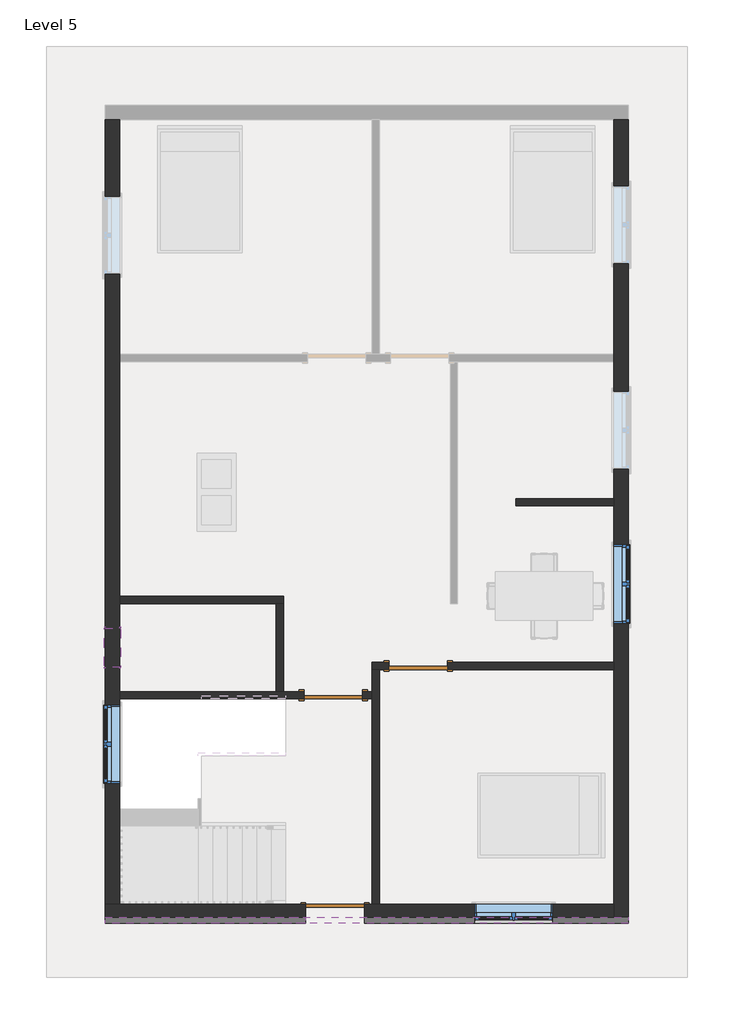
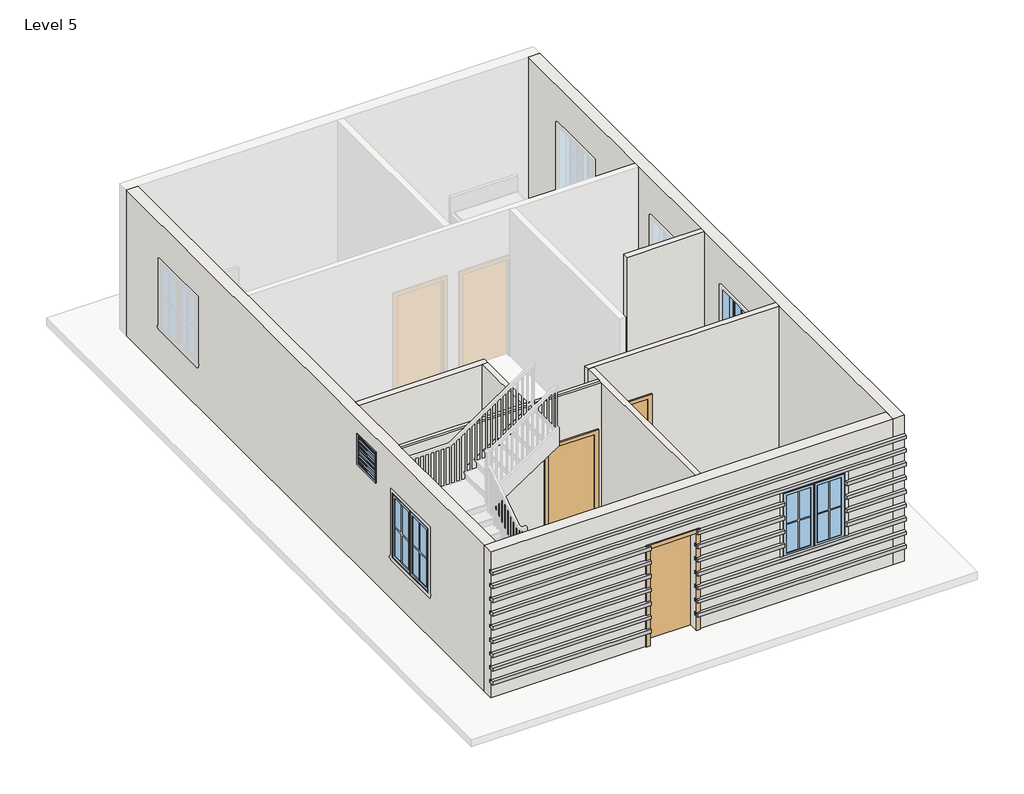
# One storey, part 1 of 3: 9 proxies, 9 walls, 4 windows, 3 doors.
"""IFC4 building model written with IfcOpenShell, lengths in millimetres."""

from ifc_helpers import new_model, si_unit, frame, origin, place, context, project, spatial, polyline, outline, extrude, faceted_brep, transform, mapped, element, save
from components import single_flush_door_3_17d80c48, single_flush_door_3_5e62189b, single_flush_door_3_89fc3733, window_casement_double_window_4_576b2d2c, window_f2d8fef0

model = new_model("IFC4")

# Units and contexts
model_context = context("Model", 3, world=origin())
ifc_project = project(units=[si_unit("LENGTHUNIT", "METRE", prefix="MILLI")], contexts=[model_context])

# Site, building, storey
site = spatial("IfcSite", under=ifc_project)
building = spatial("IfcBuilding", under=site)
storey = spatial("IfcBuildingStorey", under=building, Name="Level 5", Elevation=12649.2)

# Proxies
placement = place(None, origin())
element("IfcBuildingElementProxy", 1, Name="Reveal", ObjectType="Reveal", at=placement, inside=storey, context=model_context, shape_type="SweptSolid", body=[
    extrude(outline(polyline([(-2204.0617403, -6585.4426559), (-2204.0617403, -6677.5176559), (-5334.6117403, -6677.5176559), (-5334.6117403, -6585.4426559), (-2204.0617403, -6585.4426559)])), frame((0.0, 0.0, 12954.0), z_axis=(0.0, 0.0, 1.0), x_axis=(1.0, 0.0, 0.0)), (0.0, 0.0, 1.0), 67.7333333),
    extrude(outline(polyline([(2831.4882597, -6585.4426559), (2831.4882597, -6677.5176559), (-1289.6617403, -6677.5176559), (-1289.6617403, -6585.4426559), (2831.4882597, -6585.4426559)])), frame((0.0, 0.0, 12954.0), z_axis=(0.0, 0.0, 1.0), x_axis=(1.0, 0.0, 0.0)), (0.0, 0.0, 1.0), 67.7333333),
])
element("IfcBuildingElementProxy", 2, Name="Reveal", ObjectType="Reveal", at=placement, inside=storey, context=model_context, shape_type="SweptSolid", body=[
    extrude(outline(polyline([(-2204.0617403, -6585.4426559), (-2204.0617403, -6677.5176559), (-5334.6117403, -6677.5176559), (-5334.6117403, -6585.4426559), (-2204.0617403, -6585.4426559)])), frame((0.0, 0.0, 13240.4994231), z_axis=(0.0, 0.0, 1.0), x_axis=(1.0, 0.0, 0.0)), (0.0, 0.0, 1.0), 67.7333333),
    extrude(outline(polyline([(2831.4882597, -6585.4426559), (2831.4882597, -6677.5176559), (-1289.6617403, -6677.5176559), (-1289.6617403, -6585.4426559), (2831.4882597, -6585.4426559)])), frame((0.0, 0.0, 13240.4994231), z_axis=(0.0, 0.0, 1.0), x_axis=(1.0, 0.0, 0.0)), (0.0, 0.0, 1.0), 67.7333333),
])
element("IfcBuildingElementProxy", 3, Name="Reveal", ObjectType="Reveal", at=placement, inside=storey, context=model_context, shape_type="SweptSolid", body=[
    extrude(outline(polyline([(-2204.0617403, -6585.4426559), (-2204.0617403, -6677.5176559), (-5334.6117403, -6677.5176559), (-5334.6117403, -6585.4426559), (-2204.0617403, -6585.4426559)])), frame((0.0, 0.0, 13526.9988461), z_axis=(0.0, 0.0, 1.0), x_axis=(1.0, 0.0, 0.0)), (0.0, 0.0, 1.0), 67.7333333),
    extrude(outline(polyline([(2831.4882597, -6585.4426559), (2831.4882597, -6677.5176559), (-1289.6617403, -6677.5176559), (-1289.6617403, -6585.4426559), (2831.4882597, -6585.4426559)])), frame((0.0, 0.0, 13526.9988461), z_axis=(0.0, 0.0, 1.0), x_axis=(1.0, 0.0, 0.0)), (0.0, 0.0, 1.0), 67.7333333),
])
element("IfcBuildingElementProxy", 4, Name="Reveal", ObjectType="Reveal", at=placement, inside=storey, context=model_context, shape_type="SweptSolid", body=[
    extrude(outline(polyline([(431.1882597, -6585.4426559), (431.1882597, -6677.5176559), (-1289.6617403, -6677.5176559), (-1289.6617403, -6585.4426559), (431.1882597, -6585.4426559)])), frame((0.0, 0.0, 13813.4982692), z_axis=(0.0, 0.0, 1.0), x_axis=(1.0, 0.0, 0.0)), (0.0, 0.0, 1.0), 67.7333333),
    extrude(outline(polyline([(-2204.0617403, -6585.4426559), (-2204.0617403, -6677.5176559), (-5334.6117403, -6677.5176559), (-5334.6117403, -6585.4426559), (-2204.0617403, -6585.4426559)])), frame((0.0, 0.0, 13813.4982692), z_axis=(0.0, 0.0, 1.0), x_axis=(1.0, 0.0, 0.0)), (0.0, 0.0, 1.0), 67.7333333),
    extrude(outline(polyline([(2831.4882597, -6585.4426559), (2831.4882597, -6677.5176559), (1650.3882597, -6677.5176559), (1650.3882597, -6585.4426559), (2831.4882597, -6585.4426559)])), frame((0.0, 0.0, 13813.4982692), z_axis=(0.0, 0.0, 1.0), x_axis=(1.0, 0.0, 0.0)), (0.0, 0.0, 1.0), 67.7333333),
])
element("IfcBuildingElementProxy", 5, Name="Reveal", ObjectType="Reveal", at=placement, inside=storey, context=model_context, shape_type="SweptSolid", body=[
    extrude(outline(polyline([(431.1882597, -6585.4426559), (431.1882597, -6677.5176559), (-1289.6617403, -6677.5176559), (-1289.6617403, -6585.4426559), (431.1882597, -6585.4426559)])), frame((0.0, 0.0, 14099.9976923), z_axis=(0.0, 0.0, 1.0), x_axis=(1.0, 0.0, 0.0)), (0.0, 0.0, 1.0), 67.7333333),
    extrude(outline(polyline([(-2204.0617403, -6585.4426559), (-2204.0617403, -6677.5176559), (-5334.6117403, -6677.5176559), (-5334.6117403, -6585.4426559), (-2204.0617403, -6585.4426559)])), frame((0.0, 0.0, 14099.9976923), z_axis=(0.0, 0.0, 1.0), x_axis=(1.0, 0.0, 0.0)), (0.0, 0.0, 1.0), 67.7333333),
    extrude(outline(polyline([(2831.4882597, -6585.4426559), (2831.4882597, -6677.5176559), (1650.3882597, -6677.5176559), (1650.3882597, -6585.4426559), (2831.4882597, -6585.4426559)])), frame((0.0, 0.0, 14099.9976923), z_axis=(0.0, 0.0, 1.0), x_axis=(1.0, 0.0, 0.0)), (0.0, 0.0, 1.0), 67.7333333),
])
element("IfcBuildingElementProxy", 6, Name="Reveal", ObjectType="Reveal", at=placement, inside=storey, context=model_context, shape_type="SweptSolid", body=[
    extrude(outline(polyline([(431.1882597, -6585.4426559), (431.1882597, -6677.5176559), (-1289.6617403, -6677.5176559), (-1289.6617403, -6585.4426559), (431.1882597, -6585.4426559)])), frame((0.0, 0.0, 14386.4971154), z_axis=(0.0, 0.0, 1.0), x_axis=(1.0, 0.0, 0.0)), (0.0, 0.0, 1.0), 67.7333333),
    extrude(outline(polyline([(-2204.0617403, -6585.4426559), (-2204.0617403, -6677.5176559), (-5334.6117403, -6677.5176559), (-5334.6117403, -6585.4426559), (-2204.0617403, -6585.4426559)])), frame((0.0, 0.0, 14386.4971154), z_axis=(0.0, 0.0, 1.0), x_axis=(1.0, 0.0, 0.0)), (0.0, 0.0, 1.0), 67.7333333),
    extrude(outline(polyline([(2831.4882597, -6585.4426559), (2831.4882597, -6677.5176559), (1650.3882597, -6677.5176559), (1650.3882597, -6585.4426559), (2831.4882597, -6585.4426559)])), frame((0.0, 0.0, 14386.4971154), z_axis=(0.0, 0.0, 1.0), x_axis=(1.0, 0.0, 0.0)), (0.0, 0.0, 1.0), 67.7333333),
])
element("IfcBuildingElementProxy", 7, Name="Reveal", ObjectType="Reveal", at=placement, inside=storey, context=model_context, shape_type="SweptSolid", body=[
    extrude(outline(polyline([(431.1882597, -6585.4426559), (431.1882597, -6677.5176559), (-1289.6617403, -6677.5176559), (-1289.6617403, -6585.4426559), (431.1882597, -6585.4426559)])), frame((0.0, 0.0, 14672.9965384), z_axis=(0.0, 0.0, 1.0), x_axis=(1.0, 0.0, 0.0)), (0.0, 0.0, 1.0), 67.7333333),
    extrude(outline(polyline([(-2204.0617403, -6585.4426559), (-2204.0617403, -6677.5176559), (-5334.6117403, -6677.5176559), (-5334.6117403, -6585.4426559), (-2204.0617403, -6585.4426559)])), frame((0.0, 0.0, 14672.9965384), z_axis=(0.0, 0.0, 1.0), x_axis=(1.0, 0.0, 0.0)), (0.0, 0.0, 1.0), 67.7333333),
    extrude(outline(polyline([(2831.4882597, -6585.4426559), (2831.4882597, -6677.5176559), (1650.3882597, -6677.5176559), (1650.3882597, -6585.4426559), (2831.4882597, -6585.4426559)])), frame((0.0, 0.0, 14672.9965384), z_axis=(0.0, 0.0, 1.0), x_axis=(1.0, 0.0, 0.0)), (0.0, 0.0, 1.0), 67.7333333),
])
element("IfcBuildingElementProxy", 8, Name="Reveal", ObjectType="Reveal", at=placement, inside=storey, context=model_context, shape_type="SweptSolid", body=[
    extrude(outline(polyline([(2831.4882597, -6585.4426559), (2831.4882597, -6677.5176559), (-5334.6117403, -6677.5176559), (-5334.6117403, -6585.4426559), (2831.4882597, -6585.4426559)])), frame((0.0, 0.0, 14959.4959615), z_axis=(0.0, 0.0, 1.0), x_axis=(1.0, 0.0, 0.0)), (0.0, 0.0, 1.0), 67.7333333),
])
element("IfcBuildingElementProxy", 9, Name="Reveal", ObjectType="Reveal", at=placement, inside=storey, context=model_context, shape_type="SweptSolid", body=[
    extrude(outline(polyline([(2831.4882597, -6585.4426559), (2831.4882597, -6677.5176559), (-5334.6117403, -6677.5176559), (-5334.6117403, -6585.4426559), (2831.4882597, -6585.4426559)])), frame((0.0, 0.0, 15245.9953846), z_axis=(0.0, 0.0, 1.0), x_axis=(1.0, 0.0, 0.0)), (0.0, 0.0, 1.0), 67.7333333),
])

# Doors
single_flush_door_3_shape = single_flush_door_3_17d80c48(model_context)
element("IfcDoor", 10, ObjectType="Single-Flush : DOOR 3'", at=placement, inside=storey, context=model_context, shape_type="MappedRepresentation", body=[
    mapped(single_flush_door_3_shape, transform((-451.4617403, -2667.4926559, 12649.2), x_axis=(-1.0, 0.0, 0.0), y_axis=(0.0, -1.0, 0.0), z_axis=(0.0, 0.0, 1.0))),
])
single_flush_door_3_2_shape = single_flush_door_3_5e62189b(model_context)
element("IfcDoor", 11, ObjectType="Single-Flush : DOOR 3'", at=placement, inside=storey, context=model_context, shape_type="MappedRepresentation", body=[
    mapped(single_flush_door_3_2_shape, transform((-1772.2617403, -3124.6926559, 12649.2), x_axis=(1.0, 0.0, 0.0), y_axis=(0.0, 1.0, 0.0), z_axis=(0.0, 0.0, 1.0))),
])
single_flush_door_3_3_shape = single_flush_door_3_89fc3733(model_context)
element("IfcDoor", 12, ObjectType="Single-Flush : DOOR 3'", at=placement, inside=storey, context=model_context, shape_type="MappedRepresentation", body=[
    mapped(single_flush_door_3_3_shape, transform((-1746.8617403, -6496.5426559, 12649.2), x_axis=(1.0, 0.0, 0.0), y_axis=(0.0, 1.0, 0.0), z_axis=(0.0, 0.0, 1.0))),
])

# Walls
element("IfcWall", 13, ObjectType="ALL 4.5\"", at=placement, inside=storey, context=model_context, shape_type="SweptSolid", body=[
    extrude(outline(polyline([(1078.8882597, -57.6426559), (2602.8882597, -57.6426559), (2602.8882597, -171.9426559), (1078.8882597, -171.9426559), (1078.8882597, -57.6426559)])), frame((0.0, 0.0, 12649.2), z_axis=(0.0, 0.0, 1.0), x_axis=(1.0, 0.0, 0.0)), (0.0, 0.0, 1.0), 3048.0),
])
element("IfcWall", 14, ObjectType="ALL 4.5\"", at=placement, inside=storey, context=model_context, shape_type="Brep", body=[
    faceted_brep([(-908.6617403, -2610.3426559, 14681.2), (-908.6617403, -2610.3426559, 12649.2), (-1169.0117403, -2610.3426559, 12649.2), (-1169.0117403, -2610.3426559, 15697.2), (2602.8882597, -2610.3426559, 15697.2), (2602.8882597, -2610.3426559, 12649.2), (5.7382597, -2610.3426559, 12649.2), (5.7382597, -2610.3426559, 14681.2), (-1169.0117403, -2724.6426559, 12649.2), (-1054.7117403, -2724.6426559, 12649.2), (-908.6617403, -2724.6426559, 12649.2), (-908.6617403, -2724.6426559, 14681.2), (5.7382597, -2724.6426559, 14681.2), (5.7382597, -2724.6426559, 12649.2), (2602.8882597, -2724.6426559, 12649.2), (2602.8882597, -2724.6426559, 15697.2), (-1054.7117403, -2724.6426559, 15697.2), (-1169.0117403, -2724.6426559, 15697.2)], [[[0, 1, 2, 3, 4, 5, 6, 7]], [[8, 9, 10, 11, 12, 13, 14, 15, 16, 17]], [[6, 5, 14, 13]], [[2, 1, 10, 9, 8]], [[5, 4, 15, 14]], [[3, 2, 8, 17]], [[11, 10, 1, 0]], [[12, 11, 0, 7]], [[13, 12, 7, 6]], [[4, 3, 17, 16, 15]]]),
])
element("IfcWall", 15, ObjectType="ALL 4.5\"", at=placement, inside=storey, context=model_context, shape_type="Brep", body=[
    faceted_brep([(-1169.0117403, -2724.6426559, 12649.2), (-1169.0117403, -3067.5426559, 12649.2), (-1169.0117403, -3181.8426559, 12649.2), (-1169.0117403, -6382.2426559, 12649.2), (-1169.0117403, -6382.2426559, 15697.2), (-1169.0117403, -3181.8426559, 15697.2), (-1169.0117403, -3067.5426559, 15697.2), (-1169.0117403, -2724.6426559, 15697.2), (-1054.7117403, -2724.6426559, 12649.2), (-1054.7117403, -2724.6426559, 15697.2), (-1054.7117403, -6382.2426559, 15697.2), (-1054.7117403, -6382.2426559, 12649.2)], [[[0, 1, 2, 3, 4, 5, 6, 7]], [[8, 9, 10, 11]], [[3, 2, 1, 0, 8, 11]], [[0, 7, 9, 8]], [[4, 3, 11, 10]], [[7, 6, 5, 4, 10, 9]]]),
])
element("IfcWall", 16, ObjectType="ALL 4.5\"", at=placement, inside=storey, context=model_context, shape_type="Brep", body=[
    faceted_brep([(-1169.0117403, -3067.5426559, 12649.2), (-1315.0617403, -3067.5426559, 12649.2), (-1315.0617403, -3067.5426559, 14681.2), (-2229.4617403, -3067.5426559, 14681.2), (-2229.4617403, -3067.5426559, 12649.2), (-2553.3117403, -3067.5426559, 12649.2), (-2667.6117403, -3067.5426559, 12649.2), (-5106.0117403, -3067.5426559, 12649.2), (-5106.0117403, -3067.5426559, 15697.2), (-2667.6117403, -3067.5426559, 15697.2), (-2553.3117403, -3067.5426559, 15697.2), (-1169.0117403, -3067.5426559, 15697.2), (-1315.0617403, -3181.8426559, 14681.2), (-1315.0617403, -3181.8426559, 12649.2), (-1169.0117403, -3181.8426559, 12649.2), (-1169.0117403, -3181.8426559, 15697.2), (-5106.0117403, -3181.8426559, 15697.2), (-5106.0117403, -3181.8426559, 12649.2), (-2229.4617403, -3181.8426559, 12649.2), (-2229.4617403, -3181.8426559, 14681.2), (-5106.0117403, -3131.0426559, 15697.2), (-1169.0117403, -3131.0426559, 15697.2), (-2515.2117403, -3131.0426559, 15697.2)], [[[0, 1, 2, 3, 4, 5, 6, 7, 8, 9, 10, 11]], [[12, 13, 14, 15, 16, 17, 18, 19]], [[18, 17, 7, 6, 5, 4]], [[14, 13, 1, 0]], [[8, 7, 17, 16, 20]], [[0, 11, 21, 15, 14]], [[2, 1, 13, 12]], [[3, 2, 12, 19]], [[4, 3, 19, 18]], [[11, 10, 9, 8, 20, 22, 21]], [[20, 16, 15, 21, 22]]]),
])
element("IfcWall", 17, ObjectType="ALL 4.5\"", at=placement, inside=storey, context=model_context, shape_type="Brep", body=[
    faceted_brep([(-5106.0117403, -1695.9426559, 12649.2), (-2667.6117403, -1695.9426559, 12649.2), (-2553.3117403, -1695.9426559, 12649.2), (-2553.3117403, -1695.9426559, 15697.2), (-2667.6117403, -1695.9426559, 15697.2), (-5106.0117403, -1695.9426559, 15697.2), (-5106.0117403, -1581.6426559, 12649.2), (-5106.0117403, -1581.6426559, 15697.2), (-2553.3117403, -1581.6426559, 15697.2), (-2553.3117403, -1581.6426559, 12649.2)], [[[0, 1, 2, 3, 4, 5]], [[6, 7, 8, 9]], [[2, 1, 0, 6, 9]], [[0, 5, 7, 6]], [[3, 2, 9, 8]], [[5, 4, 3, 8, 7]]]),
])
element("IfcWall", 18, ObjectType="ALL 4.5\"", at=placement, inside=storey, context=model_context, shape_type="SweptSolid", body=[
    extrude(outline(polyline([(-2667.6117403, -3067.5426559), (-2667.6117403, -1695.9426559), (-2553.3117403, -1695.9426559), (-2553.3117403, -3067.5426559), (-2667.6117403, -3067.5426559)])), frame((0.0, 0.0, 12649.2), z_axis=(0.0, 0.0, 1.0), x_axis=(1.0, 0.0, 0.0)), (0.0, 0.0, 1.0), 3048.0),
])
element("IfcWall", 19, ObjectType="WALL 9\"", at=placement, inside=storey, context=model_context, shape_type="Brep", body=[
    faceted_brep([(2602.8882597, 5847.8573441, 12649.2), (2602.8882597, 2190.2573441, 12649.2), (2602.8882597, 2075.9573441, 12649.2), (2602.8882597, -57.6426559, 12649.2), (2602.8882597, -171.9426559, 12649.2), (2602.8882597, -2610.3426559, 12649.2), (2602.8882597, -2724.6426559, 12649.2), (2602.8882597, -6382.2426559, 12649.2), (2602.8882597, -6610.8426559, 12649.2), (2602.8882597, -6610.8426559, 12954.0), (2602.8882597, -6585.4426559, 12954.0), (2602.8882597, -6585.4426559, 13021.7333333), (2602.8882597, -6610.8426559, 13021.7333333), (2602.8882597, -6610.8426559, 13240.4994231), (2602.8882597, -6585.4426559, 13240.4994231), (2602.8882597, -6585.4426559, 13308.2327564), (2602.8882597, -6610.8426559, 13308.2327564), (2602.8882597, -6610.8426559, 13526.9988461), (2602.8882597, -6585.4426559, 13526.9988461), (2602.8882597, -6585.4426559, 13594.7321795), (2602.8882597, -6610.8426559, 13594.7321795), (2602.8882597, -6610.8426559, 13813.4982692), (2602.8882597, -6585.4426559, 13813.4982692), (2602.8882597, -6585.4426559, 13881.2316025), (2602.8882597, -6610.8426559, 13881.2316025), (2602.8882597, -6610.8426559, 14099.9976923), (2602.8882597, -6585.4426559, 14099.9976923), (2602.8882597, -6585.4426559, 14167.7310256), (2602.8882597, -6610.8426559, 14167.7310256), (2602.8882597, -6610.8426559, 14386.4971154), (2602.8882597, -6585.4426559, 14386.4971154), (2602.8882597, -6585.4426559, 14454.2304487), (2602.8882597, -6610.8426559, 14454.2304487), (2602.8882597, -6610.8426559, 14672.9965384), (2602.8882597, -6585.4426559, 14672.9965384), (2602.8882597, -6585.4426559, 14740.7298718), (2602.8882597, -6610.8426559, 14740.7298718), (2602.8882597, -6610.8426559, 14959.4959615), (2602.8882597, -6585.4426559, 14959.4959615), (2602.8882597, -6585.4426559, 15027.2292948), (2602.8882597, -6610.8426559, 15027.2292948), (2602.8882597, -6610.8426559, 15245.9953846), (2602.8882597, -6585.4426559, 15245.9953846), (2602.8882597, -6585.4426559, 15313.7287179), (2602.8882597, -6610.8426559, 15313.7287179), (2602.8882597, -6610.8426559, 15697.2), (2602.8882597, -6382.2426559, 15697.2), (2602.8882597, -2724.6426559, 15697.2), (2602.8882597, -2610.3426559, 15697.2), (2602.8882597, -171.9426559, 15697.2), (2602.8882597, -57.6426559, 15697.2), (2602.8882597, 2075.9573441, 15697.2), (2602.8882597, 2190.2573441, 15697.2), (2602.8882597, 5847.8573441, 15697.2), (2602.8882597, 3599.9573441, 14909.8), (2602.8882597, 3599.9573441, 13563.6), (2602.8882597, 4819.1573441, 13563.6), (2602.8882597, 4819.1573441, 14909.8), (2602.8882597, 399.5573441, 14909.8), (2602.8882597, 399.5573441, 13563.6), (2602.8882597, 1618.7573441, 13563.6), (2602.8882597, 1618.7573441, 14909.8), (2602.8882597, -2000.7426559, 14909.8), (2602.8882597, -2000.7426559, 13563.6), (2602.8882597, -781.5426559, 13563.6), (2602.8882597, -781.5426559, 14909.8), (2831.4882597, -6610.8426559, 12649.2), (2831.4882597, 5847.8573441, 12649.2), (2831.4882597, 5847.8573441, 15697.2), (2831.4882597, -6610.8426559, 15697.2), (2831.4882597, -6610.8426559, 15313.7287179), (2831.4882597, -6585.4426559, 15313.7287179), (2831.4882597, -6585.4426559, 15245.9953846), (2831.4882597, -6610.8426559, 15245.9953846), (2831.4882597, -6610.8426559, 15027.2292948), (2831.4882597, -6585.4426559, 15027.2292948), (2831.4882597, -6585.4426559, 14959.4959615), (2831.4882597, -6610.8426559, 14959.4959615), (2831.4882597, -6610.8426559, 14740.7298718), (2831.4882597, -6585.4426559, 14740.7298718), (2831.4882597, -6585.4426559, 14672.9965384), (2831.4882597, -6610.8426559, 14672.9965384), (2831.4882597, -6610.8426559, 14454.2304487), (2831.4882597, -6585.4426559, 14454.2304487), (2831.4882597, -6585.4426559, 14386.4971154), (2831.4882597, -6610.8426559, 14386.4971154), (2831.4882597, -6610.8426559, 14167.7310256), (2831.4882597, -6585.4426559, 14167.7310256), (2831.4882597, -6585.4426559, 14099.9976923), (2831.4882597, -6610.8426559, 14099.9976923), (2831.4882597, -6610.8426559, 13881.2316025), (2831.4882597, -6585.4426559, 13881.2316025), (2831.4882597, -6585.4426559, 13813.4982692), (2831.4882597, -6610.8426559, 13813.4982692), (2831.4882597, -6610.8426559, 13594.7321795), (2831.4882597, -6585.4426559, 13594.7321795), (2831.4882597, -6585.4426559, 13526.9988461), (2831.4882597, -6610.8426559, 13526.9988461), (2831.4882597, -6610.8426559, 13308.2327564), (2831.4882597, -6585.4426559, 13308.2327564), (2831.4882597, -6585.4426559, 13240.4994231), (2831.4882597, -6610.8426559, 13240.4994231), (2831.4882597, -6610.8426559, 13021.7333333), (2831.4882597, -6585.4426559, 13021.7333333), (2831.4882597, -6585.4426559, 12954.0), (2831.4882597, -6610.8426559, 12954.0), (2831.4882597, 3599.9573441, 13563.6), (2831.4882597, 3599.9573441, 14909.8), (2831.4882597, 4819.1573441, 14909.8), (2831.4882597, 4819.1573441, 13563.6), (2831.4882597, 399.5573441, 13563.6), (2831.4882597, 399.5573441, 14909.8), (2831.4882597, 1618.7573441, 14909.8), (2831.4882597, 1618.7573441, 13563.6), (2831.4882597, -2000.7426559, 13563.6), (2831.4882597, -2000.7426559, 14909.8), (2831.4882597, -781.5426559, 14909.8), (2831.4882597, -781.5426559, 13563.6)], [[[0, 1, 2, 3, 4, 5, 6, 7, 8, 9, 10, 11, 12, 13, 14, 15, 16, 17, 18, 19, 20, 21, 22, 23, 24, 25, 26, 27, 28, 29, 30, 31, 32, 33, 34, 35, 36, 37, 38, 39, 40, 41, 42, 43, 44, 45, 46, 47, 48, 49, 50, 51, 52, 53], [54, 55, 56, 57], [58, 59, 60, 61], [62, 63, 64, 65]], [[66, 67, 68, 69, 70, 71, 72, 73, 74, 75, 76, 77, 78, 79, 80, 81, 82, 83, 84, 85, 86, 87, 88, 89, 90, 91, 92, 93, 94, 95, 96, 97, 98, 99, 100, 101, 102, 103, 104, 105], [106, 107, 108, 109], [110, 111, 112, 113], [114, 115, 116, 117]], [[8, 7, 6, 5, 4, 3, 2, 1, 0, 67, 66]], [[0, 53, 68, 67]], [[8, 66, 105, 9]], [[69, 45, 44, 70]], [[12, 102, 101, 13]], [[16, 98, 97, 17]], [[20, 94, 93, 21]], [[24, 90, 89, 25]], [[28, 86, 85, 29]], [[32, 82, 81, 33]], [[36, 78, 77, 37]], [[40, 74, 73, 41]], [[55, 54, 107, 106]], [[56, 55, 106, 109]], [[57, 56, 109, 108]], [[54, 57, 108, 107]], [[59, 58, 111, 110]], [[60, 59, 110, 113]], [[61, 60, 113, 112]], [[58, 61, 112, 111]], [[63, 62, 115, 114]], [[64, 63, 114, 117]], [[65, 64, 117, 116]], [[62, 65, 116, 115]], [[53, 52, 51, 50, 49, 48, 47, 46, 45, 69, 68]], [[11, 103, 102, 12]], [[104, 10, 9, 105]], [[103, 11, 10, 104]], [[15, 99, 98, 16]], [[100, 14, 13, 101]], [[99, 15, 14, 100]], [[19, 95, 94, 20]], [[96, 18, 17, 97]], [[95, 19, 18, 96]], [[23, 91, 90, 24]], [[92, 22, 21, 93]], [[91, 23, 22, 92]], [[27, 87, 86, 28]], [[88, 26, 25, 89]], [[87, 27, 26, 88]], [[31, 83, 82, 32]], [[84, 30, 29, 85]], [[83, 31, 30, 84]], [[35, 79, 78, 36]], [[80, 34, 33, 81]], [[79, 35, 34, 80]], [[39, 75, 74, 40]], [[76, 38, 37, 77]], [[75, 39, 38, 76]], [[43, 71, 70, 44]], [[72, 42, 41, 73]], [[71, 43, 42, 72]]]),
])
element("IfcWall", 20, ObjectType="WALL 9\"", at=placement, inside=storey, context=model_context, shape_type="Brep", body=[
    faceted_brep([(-5334.6117403, -6382.2426559, 15697.2), (-5106.0117403, -6382.2426559, 15697.2), (-1169.0117403, -6382.2426559, 15697.2), (-1054.7117403, -6382.2426559, 15697.2), (2602.8882597, -6382.2426559, 15697.2), (2602.8882597, -6382.2426559, 12649.2), (-1054.7117403, -6382.2426559, 12649.2), (-1169.0117403, -6382.2426559, 12649.2), (-1289.6617403, -6382.2426559, 12649.2), (-1289.6617403, -6382.2426559, 14681.2), (-2204.0617403, -6382.2426559, 14681.2), (-2204.0617403, -6382.2426559, 12649.2), (-5106.0117403, -6382.2426559, 12649.2), (-5334.6117403, -6382.2426559, 12649.2), (431.1882597, -6382.2426559, 14909.8), (431.1882597, -6382.2426559, 13563.6), (1650.3882597, -6382.2426559, 13563.6), (1650.3882597, -6382.2426559, 14909.8), (2602.8882597, -6610.8426559, 15697.2), (-5334.6117403, -6610.8426559, 15697.2), (-5334.6117403, -6610.8426559, 15313.7287179), (2602.8882597, -6610.8426559, 15313.7287179), (431.1882597, -6610.8426559, 14909.8), (1650.3882597, -6610.8426559, 14909.8), (1650.3882597, -6610.8426559, 14740.7298718), (2602.8882597, -6610.8426559, 14740.7298718), (2602.8882597, -6610.8426559, 14959.4959615), (-5334.6117403, -6610.8426559, 14959.4959615), (-5334.6117403, -6610.8426559, 14740.7298718), (-2204.0617403, -6610.8426559, 14740.7298718), (-2204.0617403, -6610.8426559, 14681.2), (-1289.6617403, -6610.8426559, 14681.2), (-1289.6617403, -6610.8426559, 14740.7298718), (431.1882597, -6610.8426559, 14740.7298718), (-5334.6117403, -6610.8426559, 12954.0), (-5334.6117403, -6610.8426559, 12649.2), (-2204.0617403, -6610.8426559, 12649.2), (-2204.0617403, -6610.8426559, 12954.0), (-5334.6117403, -6610.8426559, 13021.7333333), (-2204.0617403, -6610.8426559, 13021.7333333), (-2204.0617403, -6610.8426559, 13240.4994231), (-5334.6117403, -6610.8426559, 13240.4994231), (2602.8882597, -6610.8426559, 12649.2), (2602.8882597, -6610.8426559, 12954.0), (-1289.6617403, -6610.8426559, 12954.0), (-1289.6617403, -6610.8426559, 12649.2), (-5334.6117403, -6610.8426559, 13308.2327564), (-2204.0617403, -6610.8426559, 13308.2327564), (-2204.0617403, -6610.8426559, 13526.9988461), (-5334.6117403, -6610.8426559, 13526.9988461), (2602.8882597, -6610.8426559, 13021.7333333), (2602.8882597, -6610.8426559, 13240.4994231), (-1289.6617403, -6610.8426559, 13240.4994231), (-1289.6617403, -6610.8426559, 13021.7333333), (-5334.6117403, -6610.8426559, 13594.7321795), (-2204.0617403, -6610.8426559, 13594.7321795), (-2204.0617403, -6610.8426559, 13813.4982692), (-5334.6117403, -6610.8426559, 13813.4982692), (2602.8882597, -6610.8426559, 13308.2327564), (2602.8882597, -6610.8426559, 13526.9988461), (-1289.6617403, -6610.8426559, 13526.9988461), (-1289.6617403, -6610.8426559, 13308.2327564), (431.1882597, -6610.8426559, 13594.7321795), (431.1882597, -6610.8426559, 13813.4982692), (-1289.6617403, -6610.8426559, 13813.4982692), (-1289.6617403, -6610.8426559, 13594.7321795), (1650.3882597, -6610.8426559, 13813.4982692), (1650.3882597, -6610.8426559, 13594.7321795), (2602.8882597, -6610.8426559, 13594.7321795), (2602.8882597, -6610.8426559, 13813.4982692), (-1289.6617403, -6610.8426559, 13881.2316025), (431.1882597, -6610.8426559, 13881.2316025), (431.1882597, -6610.8426559, 14099.9976923), (-1289.6617403, -6610.8426559, 14099.9976923), (-5334.6117403, -6610.8426559, 13881.2316025), (-2204.0617403, -6610.8426559, 13881.2316025), (-2204.0617403, -6610.8426559, 14099.9976923), (-5334.6117403, -6610.8426559, 14099.9976923), (1650.3882597, -6610.8426559, 14099.9976923), (1650.3882597, -6610.8426559, 13881.2316025), (2602.8882597, -6610.8426559, 13881.2316025), (2602.8882597, -6610.8426559, 14099.9976923), (-1289.6617403, -6610.8426559, 14167.7310256), (431.1882597, -6610.8426559, 14167.7310256), (431.1882597, -6610.8426559, 14386.4971154), (-1289.6617403, -6610.8426559, 14386.4971154), (-5334.6117403, -6610.8426559, 14167.7310256), (-2204.0617403, -6610.8426559, 14167.7310256), (-2204.0617403, -6610.8426559, 14386.4971154), (-5334.6117403, -6610.8426559, 14386.4971154), (1650.3882597, -6610.8426559, 14386.4971154), (1650.3882597, -6610.8426559, 14167.7310256), (2602.8882597, -6610.8426559, 14167.7310256), (2602.8882597, -6610.8426559, 14386.4971154), (-1289.6617403, -6610.8426559, 14454.2304487), (431.1882597, -6610.8426559, 14454.2304487), (431.1882597, -6610.8426559, 14672.9965384), (-1289.6617403, -6610.8426559, 14672.9965384), (-5334.6117403, -6610.8426559, 14454.2304487), (-2204.0617403, -6610.8426559, 14454.2304487), (-2204.0617403, -6610.8426559, 14672.9965384), (-5334.6117403, -6610.8426559, 14672.9965384), (1650.3882597, -6610.8426559, 14672.9965384), (1650.3882597, -6610.8426559, 14454.2304487), (2602.8882597, -6610.8426559, 14454.2304487), (2602.8882597, -6610.8426559, 14672.9965384), (-5334.6117403, -6610.8426559, 15027.2292948), (2602.8882597, -6610.8426559, 15027.2292948), (2602.8882597, -6610.8426559, 15245.9953846), (-5334.6117403, -6610.8426559, 15245.9953846), (2602.8882597, -6585.4426559, 15313.7287179), (2602.8882597, -6585.4426559, 15245.9953846), (2602.8882597, -6585.4426559, 15027.2292948), (2602.8882597, -6585.4426559, 14959.4959615), (2602.8882597, -6585.4426559, 14740.7298718), (2602.8882597, -6585.4426559, 14672.9965384), (2602.8882597, -6585.4426559, 14454.2304487), (2602.8882597, -6585.4426559, 14386.4971154), (2602.8882597, -6585.4426559, 14167.7310256), (2602.8882597, -6585.4426559, 14099.9976923), (2602.8882597, -6585.4426559, 13881.2316025), (2602.8882597, -6585.4426559, 13813.4982692), (2602.8882597, -6585.4426559, 13594.7321795), (2602.8882597, -6585.4426559, 13526.9988461), (2602.8882597, -6585.4426559, 13308.2327564), (2602.8882597, -6585.4426559, 13240.4994231), (2602.8882597, -6585.4426559, 13021.7333333), (2602.8882597, -6585.4426559, 12954.0), (-5334.6117403, -6585.4426559, 12954.0), (-5334.6117403, -6585.4426559, 13021.7333333), (-5334.6117403, -6585.4426559, 13240.4994231), (-5334.6117403, -6585.4426559, 13308.2327564), (-5334.6117403, -6585.4426559, 13526.9988461), (-5334.6117403, -6585.4426559, 13594.7321795), (-5334.6117403, -6585.4426559, 13813.4982692), (-5334.6117403, -6585.4426559, 13881.2316025), (-5334.6117403, -6585.4426559, 14099.9976923), (-5334.6117403, -6585.4426559, 14167.7310256), (-5334.6117403, -6585.4426559, 14386.4971154), (-5334.6117403, -6585.4426559, 14454.2304487), (-5334.6117403, -6585.4426559, 14672.9965384), (-5334.6117403, -6585.4426559, 14740.7298718), (-5334.6117403, -6585.4426559, 14959.4959615), (-5334.6117403, -6585.4426559, 15027.2292948), (-5334.6117403, -6585.4426559, 15245.9953846), (-5334.6117403, -6585.4426559, 15313.7287179), (431.1882597, -6585.4426559, 14740.7298718), (431.1882597, -6585.4426559, 14672.9965384), (431.1882597, -6585.4426559, 14454.2304487), (431.1882597, -6585.4426559, 14386.4971154), (431.1882597, -6585.4426559, 14167.7310256), (431.1882597, -6585.4426559, 14099.9976923), (431.1882597, -6585.4426559, 13881.2316025), (431.1882597, -6585.4426559, 13813.4982692), (431.1882597, -6585.4426559, 13594.7321795), (431.1882597, -6585.4426559, 13563.6), (1650.3882597, -6585.4426559, 13563.6), (1650.3882597, -6585.4426559, 13594.7321795), (1650.3882597, -6585.4426559, 13813.4982692), (1650.3882597, -6585.4426559, 13881.2316025), (1650.3882597, -6585.4426559, 14099.9976923), (1650.3882597, -6585.4426559, 14167.7310256), (1650.3882597, -6585.4426559, 14386.4971154), (1650.3882597, -6585.4426559, 14454.2304487), (1650.3882597, -6585.4426559, 14672.9965384), (1650.3882597, -6585.4426559, 14740.7298718), (-2204.0617403, -6585.4426559, 13021.7333333), (-2204.0617403, -6585.4426559, 12954.0), (-2204.0617403, -6585.4426559, 13308.2327564), (-2204.0617403, -6585.4426559, 13240.4994231), (-2204.0617403, -6585.4426559, 13594.7321795), (-2204.0617403, -6585.4426559, 13526.9988461), (-1289.6617403, -6585.4426559, 13881.2316025), (-1289.6617403, -6585.4426559, 13813.4982692), (-2204.0617403, -6585.4426559, 13881.2316025), (-2204.0617403, -6585.4426559, 13813.4982692), (-1289.6617403, -6585.4426559, 14167.7310256), (-1289.6617403, -6585.4426559, 14099.9976923), (-2204.0617403, -6585.4426559, 14167.7310256), (-2204.0617403, -6585.4426559, 14099.9976923), (-1289.6617403, -6585.4426559, 14454.2304487), (-1289.6617403, -6585.4426559, 14386.4971154), (-2204.0617403, -6585.4426559, 14454.2304487), (-2204.0617403, -6585.4426559, 14386.4971154), (-1289.6617403, -6585.4426559, 14681.2), (-1289.6617403, -6585.4426559, 14740.7298718), (-1289.6617403, -6585.4426559, 14672.9965384), (-2204.0617403, -6585.4426559, 14740.7298718), (-2204.0617403, -6585.4426559, 14681.2), (-2204.0617403, -6585.4426559, 14672.9965384), (-1289.6617403, -6585.4426559, 12954.0), (-1289.6617403, -6585.4426559, 13021.7333333), (-1289.6617403, -6585.4426559, 13240.4994231), (-1289.6617403, -6585.4426559, 13308.2327564), (-1289.6617403, -6585.4426559, 13526.9988461), (-1289.6617403, -6585.4426559, 13594.7321795)], [[[0, 1, 2, 3, 4, 5, 6, 7, 8, 9, 10, 11, 12, 13], [14, 15, 16, 17]], [[18, 19, 20, 21]], [[22, 23, 24, 25, 26, 27, 28, 29, 30, 31, 32, 33]], [[34, 35, 36, 37]], [[38, 39, 40, 41]], [[42, 43, 44, 45]], [[46, 47, 48, 49]], [[50, 51, 52, 53]], [[54, 55, 56, 57]], [[58, 59, 60, 61]], [[62, 63, 64, 65]], [[66, 67, 68, 69]], [[70, 71, 72, 73]], [[74, 75, 76, 77]], [[78, 79, 80, 81]], [[82, 83, 84, 85]], [[86, 87, 88, 89]], [[90, 91, 92, 93]], [[94, 95, 96, 97]], [[98, 99, 100, 101]], [[102, 103, 104, 105]], [[106, 107, 108, 109]], [[5, 42, 45, 8, 7, 6]], [[35, 13, 12, 11, 36]], [[4, 3, 2, 1, 0, 19, 18]], [[5, 4, 18, 21, 110, 111, 108, 107, 112, 113, 26, 25, 114, 115, 105, 104, 116, 117, 93, 92, 118, 119, 81, 80, 120, 121, 69, 68, 122, 123, 59, 58, 124, 125, 51, 50, 126, 127, 43, 42]], [[0, 13, 35, 34, 128, 129, 38, 41, 130, 131, 46, 49, 132, 133, 54, 57, 134, 135, 74, 77, 136, 137, 86, 89, 138, 139, 98, 101, 140, 141, 28, 27, 142, 143, 106, 109, 144, 145, 20, 19]], [[15, 14, 22, 33, 146, 147, 96, 95, 148, 149, 84, 83, 150, 151, 72, 71, 152, 153, 63, 62, 154, 155]], [[16, 15, 155, 156]], [[17, 16, 156, 157, 67, 66, 158, 159, 79, 78, 160, 161, 91, 90, 162, 163, 103, 102, 164, 165, 24, 23]], [[14, 17, 23, 22]], [[129, 166, 39, 38]], [[167, 128, 34, 37]], [[166, 129, 128, 167]], [[131, 168, 47, 46]], [[169, 130, 41, 40]], [[168, 131, 130, 169]], [[133, 170, 55, 54]], [[171, 132, 49, 48]], [[170, 133, 132, 171]], [[172, 152, 71, 70]], [[153, 173, 64, 63]], [[152, 172, 173, 153]], [[135, 174, 75, 74]], [[175, 134, 57, 56]], [[174, 135, 134, 175]], [[176, 150, 83, 82]], [[151, 177, 73, 72]], [[150, 176, 177, 151]], [[137, 178, 87, 86]], [[179, 136, 77, 76]], [[178, 137, 136, 179]], [[180, 148, 95, 94]], [[149, 181, 85, 84]], [[148, 180, 181, 149]], [[139, 182, 99, 98]], [[183, 138, 89, 88]], [[182, 139, 138, 183]], [[184, 185, 32, 31]], [[185, 146, 33, 32]], [[147, 186, 97, 96]], [[146, 185, 184, 186, 147]], [[187, 188, 30, 29]], [[141, 187, 29, 28]], [[189, 140, 101, 100]], [[187, 141, 140, 189, 188]], [[143, 112, 107, 106]], [[113, 142, 27, 26]], [[112, 143, 142, 113]], [[145, 110, 21, 20]], [[111, 144, 109, 108]], [[110, 145, 144, 111]], [[9, 8, 45, 44, 190, 191, 53, 52, 192, 193, 61, 60, 194, 195, 65, 64, 173, 172, 70, 73, 177, 176, 82, 85, 181, 180, 94, 97, 186, 184]], [[10, 9, 184, 31, 30, 188]], [[11, 10, 188, 189, 100, 99, 182, 183, 88, 87, 178, 179, 76, 75, 174, 175, 56, 55, 170, 171, 48, 47, 168, 169, 40, 39, 166, 167, 37, 36]], [[191, 126, 50, 53]], [[127, 190, 44, 43]], [[126, 191, 190, 127]], [[193, 124, 58, 61]], [[125, 192, 52, 51]], [[124, 193, 192, 125]], [[195, 154, 62, 65]], [[157, 122, 68, 67]], [[123, 194, 60, 59]], [[154, 195, 194, 123, 122, 157, 156, 155]], [[159, 120, 80, 79]], [[121, 158, 66, 69]], [[120, 159, 158, 121]], [[161, 118, 92, 91]], [[119, 160, 78, 81]], [[118, 161, 160, 119]], [[163, 116, 104, 103]], [[117, 162, 90, 93]], [[116, 163, 162, 117]], [[165, 114, 25, 24]], [[115, 164, 102, 105]], [[114, 165, 164, 115]]]),
])
element("IfcWall", 21, ObjectType="WALL 9\"", at=placement, inside=storey, context=model_context, shape_type="Brep", body=[
    faceted_brep([(-5106.0117403, -6382.2426559, 12649.2), (-5106.0117403, -3181.8426559, 12649.2), (-5106.0117403, -3067.5426559, 12649.2), (-5106.0117403, -1695.9426559, 12649.2), (-5106.0117403, -1581.6426559, 12649.2), (-5106.0117403, 2075.9573441, 12649.2), (-5106.0117403, 2190.2573441, 12649.2), (-5106.0117403, 5847.8573441, 12649.2), (-5106.0117403, 5847.8573441, 15697.2), (-5106.0117403, 2190.2573441, 15697.2), (-5106.0117403, 2075.9573441, 15697.2), (-5106.0117403, -1581.6426559, 15697.2), (-5106.0117403, -1695.9426559, 15697.2), (-5106.0117403, -3067.5426559, 15697.2), (-5106.0117403, -3181.8426559, 15697.2), (-5106.0117403, -6382.2426559, 15697.2), (-5106.0117403, -3277.0926559, 14909.8), (-5106.0117403, -3277.0926559, 13563.6), (-5106.0117403, -4496.2926559, 13563.6), (-5106.0117403, -4496.2926559, 14909.8), (-5106.0117403, 4657.2323441, 14909.8), (-5106.0117403, 4657.2323441, 13563.6), (-5106.0117403, 3438.0323441, 13563.6), (-5106.0117403, 3438.0323441, 14909.8), (-5106.0117403, -2686.5426559, 15392.4), (-5106.0117403, -2076.9426559, 15392.4), (-5106.0117403, -2076.9426559, 14782.8), (-5106.0117403, -2686.5426559, 14782.8), (-5334.6117403, -6382.2426559, 12649.2), (-5334.6117403, -6382.2426559, 15697.2), (-5334.6117403, 5847.8573441, 15697.2), (-5334.6117403, 5847.8573441, 12649.2), (-5334.6117403, -3277.0926559, 14909.8), (-5334.6117403, -4496.2926559, 14909.8), (-5334.6117403, -4496.2926559, 13563.6), (-5334.6117403, -3277.0926559, 13563.6), (-5334.6117403, 4657.2323441, 14909.8), (-5334.6117403, 3438.0323441, 14909.8), (-5334.6117403, 3438.0323441, 13563.6), (-5334.6117403, 4657.2323441, 13563.6), (-5334.6117403, -2686.5426559, 15392.4), (-5334.6117403, -2686.5426559, 14782.8), (-5334.6117403, -2076.9426559, 14782.8), (-5334.6117403, -2076.9426559, 15392.4)], [[[0, 1, 2, 3, 4, 5, 6, 7, 8, 9, 10, 11, 12, 13, 14, 15], [16, 17, 18, 19], [20, 21, 22, 23], [24, 25, 26, 27]], [[28, 29, 30, 31], [32, 33, 34, 35], [36, 37, 38, 39], [40, 41, 42, 43]], [[7, 6, 5, 4, 3, 2, 1, 0, 28, 31]], [[15, 14, 13, 12, 11, 10, 9, 8, 30, 29]], [[8, 7, 31, 30]], [[0, 15, 29, 28]], [[17, 16, 32, 35]], [[18, 17, 35, 34]], [[19, 18, 34, 33]], [[16, 19, 33, 32]], [[21, 20, 36, 39]], [[22, 21, 39, 38]], [[23, 22, 38, 37]], [[20, 23, 37, 36]], [[41, 40, 24, 27]], [[42, 41, 27, 26]], [[43, 42, 26, 25]], [[40, 43, 25, 24]]]),
])

# Windows
window_casement_double_window_4_shape = window_casement_double_window_4_576b2d2c(model_context)
element("IfcWindow", 22, ObjectType="Window-Casement-Double : WINDOW 4'", at=placement, inside=storey, context=model_context, shape_type="MappedRepresentation", body=[
    mapped(window_casement_double_window_4_shape, transform((-5220.3117403, -3886.6926559, 12649.2), x_axis=(0.0, 1.0, 0.0), y_axis=(-1.0, 0.0, 0.0), z_axis=(0.0, 0.0, 1.0))),
])
element("IfcWindow", 23, ObjectType="Window-Casement-Double : WINDOW 4'", at=placement, inside=storey, context=model_context, shape_type="MappedRepresentation", body=[
    mapped(window_casement_double_window_4_shape, transform((2717.1882597, -1391.1426559, 12649.2), x_axis=(0.0, -1.0, 0.0), y_axis=(1.0, 0.0, 0.0), z_axis=(0.0, 0.0, 1.0))),
])
element("IfcWindow", 24, ObjectType="Window-Casement-Double : WINDOW 4'", at=placement, inside=storey, context=model_context, shape_type="MappedRepresentation", body=[
    mapped(window_casement_double_window_4_shape, transform((1040.7882597, -6496.5426559, 12649.2), x_axis=(-1.0, 0.0, 0.0), y_axis=(0.0, -1.0, 0.0), z_axis=(0.0, 0.0, 1.0))),
])
window_shape = window_f2d8fef0(model_context)
element("IfcWindow", 25, ObjectType="Window-Louvers : 24\" x 24\"", at=placement, inside=storey, context=model_context, shape_type="MappedRepresentation", body=[
    mapped(window_shape, transform((-5226.6617403, -2381.7426559, 13868.4), x_axis=(0.0, 1.0, 0.0), y_axis=(-1.0, 0.0, 0.0), z_axis=(0.0, 0.0, 1.0))),
])

save(model, "model.ifc")

# Revit data of these elements
# Type "Single-Flush : DOOR 3'"
#   Type Mark = "8"
#   Construction Type Id = "MDOOR"
#   Assembly Code = "C1020"
#   Analytic Construction = "Metal"
#   Thickness = 0' - 2"
#   Heat Transfer Coefficient (U) = 0.651978 BTU/(h·ft²·°F)
#   Height = 6' - 8"
#   Trim Projection Ext = 0' - 1"
#   Trim Projection Int = 0' - 1"
#   Trim Width = 0' - 3"
#   Width = 3' - 0"
#   Define Thermal Properties by = 1
#   Door Material = Door - Panel
#   Frame Material = Door - Frame
#   Visual Light Transmittance = 0
#   Solar Heat Gain Coefficient = 0
#   Function = (empty or 0)
#   Wall Closure = (empty or 0)
# Type "ALL 4.5\""
#   Assembly Code = "B2010"
#   Layers, outside or top first: 0' - 4 1/2" no material (function 1)
# Type "WALL 9\""
#   Assembly Code = "B2010"
#   Layers, outside or top first: 0' - 9" "Carpet (1)" (function 1)
# Type "Window-Casement-Double : WINDOW 4'"
#   Type Mark = "18"
#   Fire Rating = "0.5h"
#   Assembly Code = "B2020100"
#   Analytic Construction = "Double glazing - domestic"
#   Frame Extension [instance default] = 0' - 0 1/4"
#   Window Inset [instance default] = 0' - 0"
#   Wall Thickness [instance default] = 0' - 6"
#   Interior Wall Closure [instance default] = 0' - 2 1/4"
#   Half Width = 2' - 0"
#   Visual Light Transmittance = 0.81
#   Thermal Resistance (R) = 1.8146 (h·ft²·°F)/BTU
#   Solar Heat Gain Coefficient = 0.76
#   Rough Width = 4' - 0 1/2"
#   Rough Height = 4' - 5 1/2"
#   Height = 4' - 5"
#   Heat Transfer Coefficient (U) = 0.5511 BTU/(h·ft²·°F)
#   Exterior Wall Closure [instance default] = 0' - 1 1/4"
#   Extension Jamb [instance default] = 0' - 2 1/4"
#   Default Sill Height = 3' - 0"
#   Width = 4' - 0"
#   Muntin Visibility = yes
#   Interior Trim Visibility [instance default] = yes
#   Exterior Trim Visibility [instance default] = yes
#   Extension Jamb Visibility [instance default] = yes
#   Interior Trim Material = Wood - Stained
#   Muntin Pattern = Muntin Pattern_2x2 : Muntin Pattern_2x2
#   Interior Trim = Trim-Window-Interior-Flat : Picture Frame
#   Interior Frame Material = Wood - Stained
#   Glass Panel Material = Glass
#   Exterior Trim Material = Clad - White
#   Exterior Trim = Trim-Window-Exterior-Flat : with Sill
#   Exterior Frame Material = Clad - White
#   Wall Closure = (empty or 0)
# Type "Window-Louvers : 24\" x 24\""
#   Type Mark = "19"
#   Construction Type Id = "GSP4R"
#   Assembly Code = "B20"
#   Analytic Construction = "1/8 in Pilkington single glazing"
#   Visual Light Transmittance = 0.9
#   Thermal Resistance (R) = 1.53941 (h·ft²·°F)/BTU
#   Solar Heat Gain Coefficient = 0.78
#   Max Height = 1' - 11.74264"
#   Height = 2' - 0"
#   Heat Transfer Coefficient (U) = 0.6496 BTU/(h·ft²·°F)
#   Blade Width [instance default] = 1' - 10 1/2"
#   Blade Vertical Thickness = 0' - 0.35355"
#   Blade Thickness = 0' - 0 1/4"
#   Blade Spacing = 0' - 1 1/2"
#   Blade Height = 0' - 1.85355"
#   Blade Depth = 0' - 3"
#   Blade Angle = 45.00°
#   Default Sill Height = 3' - 0"
#   Trim Projection_Exterior = 0' - 0 1/2"
#   Trim Projection_Interior = 0' - 0 1/2"
#   Trim Width_Exterior = 0' - 1 1/2"
#   Trim Width_Interior = 0' - 1 1/2"
#   Width = 2' - 0"
#   Max Blade Count = 12
#   Define Thermal Properties by = 1
#   Blade Count = 12
#   Frame Material = Birch
#   Louver Material = Birch
#   Trim Exterior Material = Birch
#   Trim Interior Material = Birch
#   Wall Closure = (empty or 0)
# Elements 10, 11, 12 (IfcDoor, "Single-Flush : DOOR 3'")
#   Phase Created = New Construction
#   Materials on its faces: "Door - Frame", "Door - Panel"
# Elements 13, 17, 18 (IfcWall, "ALL 4.5\"")
#   Top Offset = 0' - 0"
#   Base Offset = 0' - 0"
#   Unconnected Height = 10' - 0"
#   wall height = 10' - 0"
#   Phase Created = New Construction
#   Base Constraint = Level 5
#   Materials on its faces: "Default Wall"
# Elements 14, 15, 16 (IfcWall, "ALL 4.5\"")
#   Top Offset = 0' - 0"
#   Base Offset = 0' - 0"
#   Unconnected Height = 10' - 0"
#   wall height = 10' - 0"
#   Phase Created = New Construction
#   Base Constraint = Level 5
#   Materials on its faces: "Default Wall", "Clad - White"
# Element 19 (IfcWall, "WALL 9\"")
#   Top Offset = 0' - 0"
#   Base Offset = 0' - 0"
#   Unconnected Height = 10' - 0"
#   wall height = 10' - 0"
#   Phase Created = New Construction
#   Base Constraint = Level 5
#   Materials on its faces: "Carpet (1)", "Wood - Stained"
# Elements 20, 21 (IfcWall, "WALL 9\"")
#   Top Offset = 0' - 0"
#   Base Offset = 0' - 0"
#   Unconnected Height = 10' - 0"
#   wall height = 10' - 0"
#   Phase Created = New Construction
#   Base Constraint = Level 5
#   Materials on its faces: "Carpet (1)", "Clad - White", "Wood - Stained"
# Element 22 (IfcWindow, "Window-Casement-Double : WINDOW 4'")
#   Mark = "29"
#   Window Inset = 0' - 0"
#   Interior Wall Closure = 0' - 2 1/4"
#   Frame Extension = 0' - 0 1/4"
#   Exterior Wall Closure = 0' - 1 1/4"
#   Interior Trim Visibility = yes
#   Exterior Trim Visibility = yes
#   Phase Created = New Construction
#   Materials on its faces: "Wood - Stained", "Glass", "Clad - White"
# Element 23 (IfcWindow, "Window-Casement-Double : WINDOW 4'")
#   Mark = "33"
#   Window Inset = 0' - 0"
#   Interior Wall Closure = 0' - 2 1/4"
#   Frame Extension = 0' - 0 1/4"
#   Exterior Wall Closure = 0' - 1 1/4"
#   Interior Trim Visibility = yes
#   Exterior Trim Visibility = yes
#   Phase Created = New Construction
#   Materials on its faces: "Wood - Stained", "Glass", "Clad - White"
# Element 24 (IfcWindow, "Window-Casement-Double : WINDOW 4'")
#   Mark = "34"
#   Window Inset = 0' - 0"
#   Interior Wall Closure = 0' - 2 1/4"
#   Frame Extension = 0' - 0 1/4"
#   Exterior Wall Closure = 0' - 1 1/4"
#   Interior Trim Visibility = yes
#   Exterior Trim Visibility = yes
#   Phase Created = New Construction
#   Materials on its faces: "Wood - Stained", "Glass", "Clad - White"
# Element 25 (IfcWindow, "Window-Louvers : 24\" x 24\"")
#   Mark = "35"
#   Blade Width = 1' - 10 1/2"
#   Phase Created = New Construction
#   Materials on its faces: "Birch"
# Materials
#   "Door - Panel": class "Wood", colour RGB 210 159 95, transparency 0, Cost = 0
#   "Door - Frame": colour RGB 118 70 51, transparency 0, Cost = 0
#   "Carpet (1)": class "Carpet", colour RGB 124 80 67, transparency 0, Description = "Interior finish", Cost = 0
#   "Wood - Stained": class "Wood", colour RGB 224 178 126, transparency 0, Cost = 0
#   "Glass": class "Glass", colour RGB 0 128 192, transparency 0.75, Description = "Soda Lime Glass", Cost = 0
#   "Clad - White": class "Wood", colour RGB 242 242 238, transparency 0, Cost = 0
#   "Birch": class "Wood", colour RGB 224 178 126, transparency 0, Description = "Betula Alleghaniensis", Cost = 0
#   "Default Wall": colour RGB 128 128 128, transparency 0, Cost = 0
